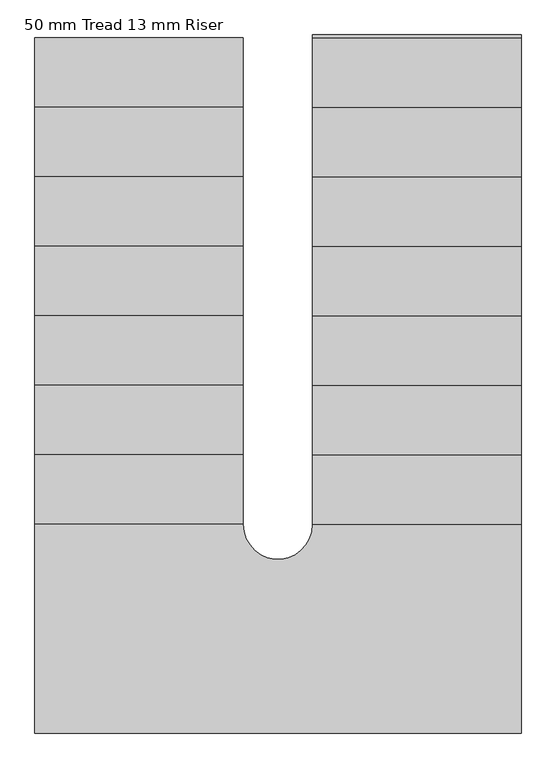
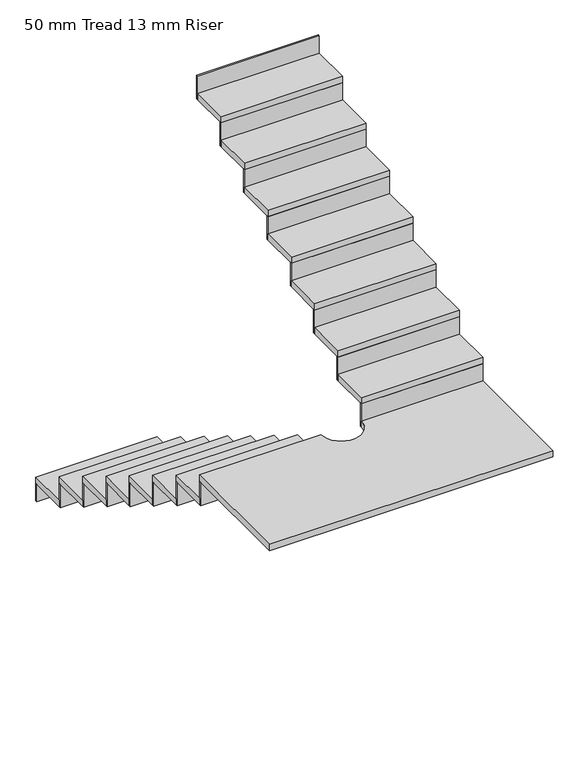
"""IFC4 building model written with IfcOpenShell, lengths in millimetres: stair flight geometry, 50 mm Tread 13 mm Riser."""

from ifc_helpers import new_model, si_unit, point, frame, frame_2d, origin, origin_with_axes, place, context, project, spatial, polyline, circle_curve, trimmed, segment, composite_curve, outline, extrude, source, transform, mapped, element, save


def stair_flight_50_mm_tread_13_mm_riser_8b475ff7(model_context):
    return source(origin(), model_context, "Body", "SweptSolid", [
        extrude(outline(polyline([(-7548.7089855, 9090.615953), (-7548.7089855, 9103.115953), (-6634.3089855, 9103.115953), (-6634.3089855, 9090.615953), (-7548.7089855, 9090.615953)])), origin_with_axes(), (0.0, 0.0, 1.0), 137.5),
        extrude(outline(polyline([(-6634.3089855, 8798.315953), (-7548.7089855, 8798.315953), (-7548.7089855, 9103.115953), (-6634.3089855, 9103.115953), (-6634.3089855, 8798.315953)])), frame((0.0, 0.0, 137.5), z_axis=(0.0, 0.0, 1.0), x_axis=(1.0, 0.0, 0.0)), (0.0, 0.0, 1.0), 50.0),
        extrude(outline(polyline([(-7548.7089855, 8785.815953), (-7548.7089855, 8798.315953), (-6634.3089855, 8798.315953), (-6634.3089855, 8785.815953), (-7548.7089855, 8785.815953)])), frame((0.0, 0.0, 137.5), z_axis=(0.0, 0.0, 1.0), x_axis=(1.0, 0.0, 0.0)), (0.0, 0.0, 1.0), 187.5),
        extrude(outline(polyline([(-6634.3089855, 8493.515953), (-7548.7089855, 8493.515953), (-7548.7089855, 8798.315953), (-6634.3089855, 8798.315953), (-6634.3089855, 8493.515953)])), frame((0.0, 0.0, 325.0), z_axis=(0.0, 0.0, 1.0), x_axis=(1.0, 0.0, 0.0)), (0.0, 0.0, 1.0), 50.0),
        extrude(outline(polyline([(-7548.7089855, 8481.015953), (-7548.7089855, 8493.515953), (-6634.3089855, 8493.515953), (-6634.3089855, 8481.015953), (-7548.7089855, 8481.015953)])), frame((0.0, 0.0, 325.0), z_axis=(0.0, 0.0, 1.0), x_axis=(1.0, 0.0, 0.0)), (0.0, 0.0, 1.0), 187.5),
        extrude(outline(polyline([(-6634.3089855, 8188.715953), (-7548.7089855, 8188.715953), (-7548.7089855, 8493.515953), (-6634.3089855, 8493.515953), (-6634.3089855, 8188.715953)])), frame((0.0, 0.0, 512.5), z_axis=(0.0, 0.0, 1.0), x_axis=(1.0, 0.0, 0.0)), (0.0, 0.0, 1.0), 50.0),
        extrude(outline(polyline([(-7548.7089855, 8176.215953), (-7548.7089855, 8188.715953), (-6634.3089855, 8188.715953), (-6634.3089855, 8176.215953), (-7548.7089855, 8176.215953)])), frame((0.0, 0.0, 512.5), z_axis=(0.0, 0.0, 1.0), x_axis=(1.0, 0.0, 0.0)), (0.0, 0.0, 1.0), 187.5),
        extrude(outline(polyline([(-6634.3089855, 7883.915953), (-7548.7089855, 7883.915953), (-7548.7089855, 8188.715953), (-6634.3089855, 8188.715953), (-6634.3089855, 7883.915953)])), frame((0.0, 0.0, 700.0), z_axis=(0.0, 0.0, 1.0), x_axis=(1.0, 0.0, 0.0)), (0.0, 0.0, 1.0), 50.0),
        extrude(outline(polyline([(-7548.7089855, 7871.415953), (-7548.7089855, 7883.915953), (-6634.3089855, 7883.915953), (-6634.3089855, 7871.415953), (-7548.7089855, 7871.415953)])), frame((0.0, 0.0, 700.0), z_axis=(0.0, 0.0, 1.0), x_axis=(1.0, 0.0, 0.0)), (0.0, 0.0, 1.0), 187.5),
        extrude(outline(polyline([(-6634.3089855, 7579.115953), (-7548.7089855, 7579.115953), (-7548.7089855, 7883.915953), (-6634.3089855, 7883.915953), (-6634.3089855, 7579.115953)])), frame((0.0, 0.0, 887.5), z_axis=(0.0, 0.0, 1.0), x_axis=(1.0, 0.0, 0.0)), (0.0, 0.0, 1.0), 50.0),
        extrude(outline(polyline([(-7548.7089855, 7566.615953), (-7548.7089855, 7579.115953), (-6634.3089855, 7579.115953), (-6634.3089855, 7566.615953), (-7548.7089855, 7566.615953)])), frame((0.0, 0.0, 887.5), z_axis=(0.0, 0.0, 1.0), x_axis=(1.0, 0.0, 0.0)), (0.0, 0.0, 1.0), 187.5),
        extrude(outline(polyline([(-6634.3089855, 7274.315953), (-7548.7089855, 7274.315953), (-7548.7089855, 7579.115953), (-6634.3089855, 7579.115953), (-6634.3089855, 7274.315953)])), frame((0.0, 0.0, 1075.0), z_axis=(0.0, 0.0, 1.0), x_axis=(1.0, 0.0, 0.0)), (0.0, 0.0, 1.0), 50.0),
        extrude(outline(polyline([(-7548.7089855, 7261.815953), (-7548.7089855, 7274.315953), (-6634.3089855, 7274.315953), (-6634.3089855, 7261.815953), (-7548.7089855, 7261.815953)])), frame((0.0, 0.0, 1075.0), z_axis=(0.0, 0.0, 1.0), x_axis=(1.0, 0.0, 0.0)), (0.0, 0.0, 1.0), 187.5),
        extrude(outline(polyline([(-6634.3089855, 6969.515953), (-7548.7089855, 6969.515953), (-7548.7089855, 7274.315953), (-6634.3089855, 7274.315953), (-6634.3089855, 6969.515953)])), frame((0.0, 0.0, 1262.5), z_axis=(0.0, 0.0, 1.0), x_axis=(1.0, 0.0, 0.0)), (0.0, 0.0, 1.0), 50.0),
        extrude(outline(composite_curve([segment(polyline([(-7548.7089855, 6957.015953), (-7548.7089855, 6969.515953), (-6634.3089855, 6969.515953)]), True, "CONTINUOUS"), segment(trimmed(circle_curve(frame_2d((-6481.9089855, 6969.515953)), 152.4), [point((-6634.3089855, 6969.515953))], [point((-6633.7954892, 6957.015953))], True, "CARTESIAN"), True, "CONTINUOUS"), segment(polyline([(-6633.7954892, 6957.015953), (-7548.7089855, 6957.015953)]), True, "CONTINUOUS")], self_intersect=False)), frame((0.0, 0.0, 1262.5), z_axis=(0.0, 0.0, 1.0), x_axis=(1.0, 0.0, 0.0)), (0.0, 0.0, 1.0), 187.5),
        extrude(outline(composite_curve([segment(polyline([(-6329.5089855, 6969.515953), (-5415.1089855, 6969.515953), (-5415.1089855, 6055.115953), (-7548.7089855, 6055.115953), (-7548.7089855, 6969.515953), (-6634.3089855, 6969.515953)]), True, "CONTINUOUS"), segment(trimmed(circle_curve(frame_2d((-6481.9089855, 6969.515953)), 152.4), [point((-6634.3089855, 6969.515953))], [point((-6329.5089855, 6969.515953))], True, "CARTESIAN"), True, "CONTINUOUS")], self_intersect=False)), frame((0.0, 0.0, 1450.0), z_axis=(0.0, 0.0, 1.0), x_axis=(1.0, 0.0, 0.0)), (0.0, 0.0, 1.0), 50.0),
        extrude(outline(polyline([(-5415.1089855, 6982.015953), (-5415.1089855, 6969.515953), (-6329.5089855, 6969.515953), (-6329.5089855, 6982.015953), (-5415.1089855, 6982.015953)])), frame((0.0, 0.0, 1450.0), z_axis=(0.0, 0.0, 1.0), x_axis=(1.0, 0.0, 0.0)), (0.0, 0.0, 1.0), 187.5),
        extrude(outline(polyline([(-6329.5089855, 7274.315953), (-5415.1089855, 7274.315953), (-5415.1089855, 6969.515953), (-6329.5089855, 6969.515953), (-6329.5089855, 7274.315953)])), frame((0.0, 0.0, 1637.5), z_axis=(0.0, 0.0, 1.0), x_axis=(1.0, 0.0, 0.0)), (0.0, 0.0, 1.0), 50.0),
        extrude(outline(polyline([(-5415.1089855, 7286.815953), (-5415.1089855, 7274.315953), (-6329.5089855, 7274.315953), (-6329.5089855, 7286.815953), (-5415.1089855, 7286.815953)])), frame((0.0, 0.0, 1637.5), z_axis=(0.0, 0.0, 1.0), x_axis=(1.0, 0.0, 0.0)), (0.0, 0.0, 1.0), 187.5),
        extrude(outline(polyline([(-6329.5089855, 7579.115953), (-5415.1089855, 7579.115953), (-5415.1089855, 7274.315953), (-6329.5089855, 7274.315953), (-6329.5089855, 7579.115953)])), frame((0.0, 0.0, 1825.0), z_axis=(0.0, 0.0, 1.0), x_axis=(1.0, 0.0, 0.0)), (0.0, 0.0, 1.0), 50.0),
        extrude(outline(polyline([(-5415.1089855, 7591.615953), (-5415.1089855, 7579.115953), (-6329.5089855, 7579.115953), (-6329.5089855, 7591.615953), (-5415.1089855, 7591.615953)])), frame((0.0, 0.0, 1825.0), z_axis=(0.0, 0.0, 1.0), x_axis=(1.0, 0.0, 0.0)), (0.0, 0.0, 1.0), 187.5),
        extrude(outline(polyline([(-6329.5089855, 7883.915953), (-5415.1089855, 7883.915953), (-5415.1089855, 7579.115953), (-6329.5089855, 7579.115953), (-6329.5089855, 7883.915953)])), frame((0.0, 0.0, 2012.5), z_axis=(0.0, 0.0, 1.0), x_axis=(1.0, 0.0, 0.0)), (0.0, 0.0, 1.0), 50.0),
        extrude(outline(polyline([(-5415.1089855, 7896.415953), (-5415.1089855, 7883.915953), (-6329.5089855, 7883.915953), (-6329.5089855, 7896.415953), (-5415.1089855, 7896.415953)])), frame((0.0, 0.0, 2012.5), z_axis=(0.0, 0.0, 1.0), x_axis=(1.0, 0.0, 0.0)), (0.0, 0.0, 1.0), 187.5),
        extrude(outline(polyline([(-6329.5089855, 8188.715953), (-5415.1089855, 8188.715953), (-5415.1089855, 7883.915953), (-6329.5089855, 7883.915953), (-6329.5089855, 8188.715953)])), frame((0.0, 0.0, 2200.0), z_axis=(0.0, 0.0, 1.0), x_axis=(1.0, 0.0, 0.0)), (0.0, 0.0, 1.0), 50.0),
        extrude(outline(polyline([(-5415.1089855, 8201.215953), (-5415.1089855, 8188.715953), (-6329.5089855, 8188.715953), (-6329.5089855, 8201.215953), (-5415.1089855, 8201.215953)])), frame((0.0, 0.0, 2200.0), z_axis=(0.0, 0.0, 1.0), x_axis=(1.0, 0.0, 0.0)), (0.0, 0.0, 1.0), 187.5),
        extrude(outline(polyline([(-6329.5089855, 8493.515953), (-5415.1089855, 8493.515953), (-5415.1089855, 8188.715953), (-6329.5089855, 8188.715953), (-6329.5089855, 8493.515953)])), frame((0.0, 0.0, 2387.5), z_axis=(0.0, 0.0, 1.0), x_axis=(1.0, 0.0, 0.0)), (0.0, 0.0, 1.0), 50.0),
        extrude(outline(polyline([(-5415.1089855, 8506.015953), (-5415.1089855, 8493.515953), (-6329.5089855, 8493.515953), (-6329.5089855, 8506.015953), (-5415.1089855, 8506.015953)])), frame((0.0, 0.0, 2387.5), z_axis=(0.0, 0.0, 1.0), x_axis=(1.0, 0.0, 0.0)), (0.0, 0.0, 1.0), 187.5),
        extrude(outline(polyline([(-6329.5089855, 8798.315953), (-5415.1089855, 8798.315953), (-5415.1089855, 8493.515953), (-6329.5089855, 8493.515953), (-6329.5089855, 8798.315953)])), frame((0.0, 0.0, 2575.0), z_axis=(0.0, 0.0, 1.0), x_axis=(1.0, 0.0, 0.0)), (0.0, 0.0, 1.0), 50.0),
        extrude(outline(polyline([(-5415.1089855, 8810.815953), (-5415.1089855, 8798.315953), (-6329.5089855, 8798.315953), (-6329.5089855, 8810.815953), (-5415.1089855, 8810.815953)])), frame((0.0, 0.0, 2575.0), z_axis=(0.0, 0.0, 1.0), x_axis=(1.0, 0.0, 0.0)), (0.0, 0.0, 1.0), 187.5),
        extrude(outline(polyline([(-5415.1089855, 9115.615953), (-5415.1089855, 9103.115953), (-6329.5089855, 9103.115953), (-6329.5089855, 9115.615953), (-5415.1089855, 9115.615953)])), frame((0.0, 0.0, 2762.5), z_axis=(0.0, 0.0, 1.0), x_axis=(1.0, 0.0, 0.0)), (0.0, 0.0, 1.0), 187.5),
        extrude(outline(polyline([(-6329.5089855, 9103.115953), (-5415.1089855, 9103.115953), (-5415.1089855, 8798.315953), (-6329.5089855, 8798.315953), (-6329.5089855, 9103.115953)])), frame((0.0, 0.0, 2762.5), z_axis=(0.0, 0.0, 1.0), x_axis=(1.0, 0.0, 0.0)), (0.0, 0.0, 1.0), 50.0),
    ])


if __name__ == "__main__":
    model = new_model("IFC4")
    model_context = context("Model", 3, world=origin())
    ifc_project = project(units=[si_unit("LENGTHUNIT", "METRE", prefix="MILLI")], contexts=[model_context])
    site = spatial("IfcSite", under=ifc_project)
    building = spatial("IfcBuilding", under=site)
    placement = place(None, origin())
    stair_flight_50_mm_tread_13_mm_riser_shape = stair_flight_50_mm_tread_13_mm_riser_8b475ff7(model_context)
    element("IfcStairFlight", 1, ObjectType="50 mm Tread 13 mm Riser", at=placement, inside=building, context=model_context, shape_type="MappedRepresentation", body=[
        mapped(stair_flight_50_mm_tread_13_mm_riser_shape, transform((0.0, 0.0, 0.0), x_axis=(1.0, 0.0, 0.0), y_axis=(0.0, 1.0, 0.0), z_axis=(0.0, 0.0, 1.0))),
    ])
    save(model, "model.ifc")
